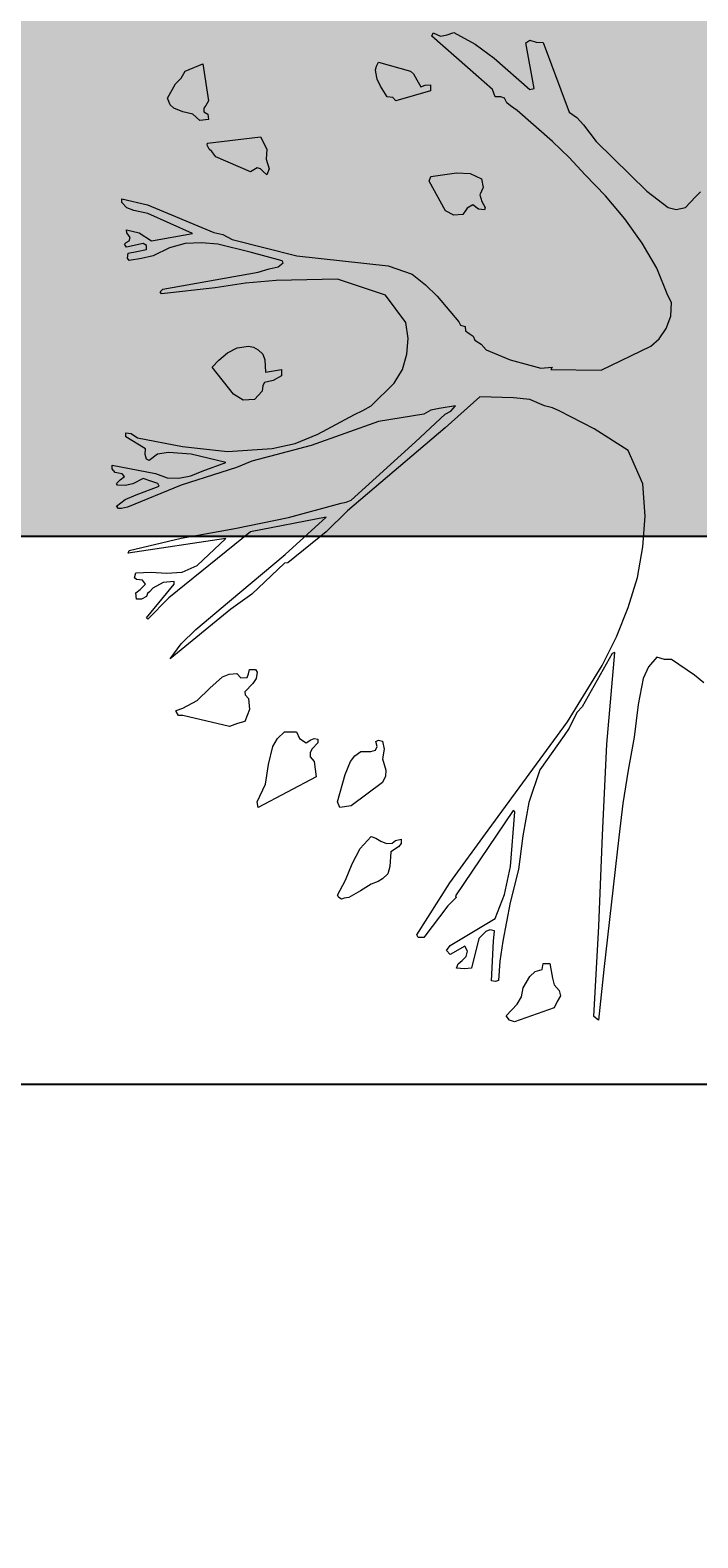
# Model space of a CAD drawing. Units: inches. Extents: x 84 to 1044, y -280 to 906.
# Tile 27 of 105: x 764 to 775, y -129 to -105. Entities that reach past the tile are written whole.
import ezdxf

# ---------------------------------------------------------------- set-up
doc = ezdxf.new("R2010")
doc.units = ezdxf.units.IN
for name, color, linetype, lineweight in [('A-ANNO-DIMS', 2, 'Continuous', 18), ('C-PROP', 7, 'Continuous', 25), ('L-PLNT', 114, 'Continuous', 15)]:
    doc.layers.add(name, color=color, linetype=linetype, lineweight=lineweight)
doc.layers.add('L-PLNT-PATT', color=9, linetype='Continuous', lineweight=9, true_color=0xafd9aa)
doc.styles.get("Standard").update_dxf_attribs({"font": 'arial.ttf'})
doc.dimstyles.get("Standard").update_dxf_attribs({"dimtxt": 0.18, "dimasz": 0.18, "dimexe": 0.18, "dimexo": 0.0625, "dimgap": 0.09, "dimtad": 0, "dimtih": 1, "dimtoh": 1, "dimdec": 4, "dimzin": 0, "dimdsep": 46, "dimtxsty": 'Standard', "dimcen": 0.09, "dimadec": 0, "dimazin": 0, "dimtfac": 1, "dimtdec": 4, "dimtofl": 0, "dimtmove": 0, "dimatfit": 3, "dimfxl": 1, "dimtolj": 1, "dimtzin": 0, "dimarcsym": 0})

# ---------------------------------------------------------------- blocks, each defined once
blk = doc.blocks.new('A$C37E508DF')
for p, q in [((0.3456, 1.093), (0.3469, 1.0964)), ((0.3842, 1.0591), (0.3456, 1.093)), ((0.3469, 1.0964), (0.355, 1.093)), ((0.355, 1.093), (0.3619, 1.0943)), ((0.3619, 1.0943), (0.3692, 1.0968)), ((0.3692, 1.0968), (0.3923, 1.0844)), ((0.3923, 1.0844), (0.4129, 1.069)), ((0.4472, 1.0857), (0.4515, 1.0887)), ((0.4562, 1.0364), (0.4472, 1.0857)), ((0.4515, 1.0887), (0.4584, 1.0865)), ((0.4584, 1.0865), (0.4657, 1.0861)), ((0.4657, 1.0861), (0.4939, 1.0107)), ((0.0789, 1.0552), (0.0978, 1.063)), ((0.0978, 1.063), (0.1042, 1.0231)), ((0.2847, 1.0565), (0.2856, 1.0604)), ((0.2856, 1.0604), (0.2877, 1.0647)), ((0.2877, 1.0647), (0.3224, 1.0552)), ((0.4129, 1.069), (0.4515, 1.0351)), ((0.0682, 1.0415), (0.0746, 1.0475)), ((0.0746, 1.0475), (0.0789, 1.0552)), ((0.2851, 1.054), (0.2847, 1.0565)), ((0.2864, 1.0463), (0.2851, 1.054)), ((0.2899, 1.039), (0.2864, 1.0463)), ((0.3224, 1.0552), (0.3255, 1.0522)), ((0.3255, 1.0522), (0.3293, 1.0458)), ((0.3293, 1.0458), (0.3336, 1.0381)), ((0.4112, 1.0351), (0.3842, 1.0591)), ((0.0596, 1.0257), (0.0682, 1.0415)), ((0.2972, 1.0274), (0.2899, 1.039)), ((0.3032, 1.0265), (0.2972, 1.0274)), ((0.3439, 1.0338), (0.3066, 1.0231)), ((0.3336, 1.0381), (0.3383, 1.0398)), ((0.3383, 1.0398), (0.3439, 1.0402)), ((0.3439, 1.0402), (0.3439, 1.0338)), ((0.4138, 1.0274), (0.4112, 1.0351)), ((0.4202, 1.0274), (0.4138, 1.0274)), ((0.4241, 1.0257), (0.4202, 1.0274)), ((0.4515, 1.0351), (0.4562, 1.0364)), ((0.0626, 1.0188), (0.0596, 1.0257)), ((0.0665, 1.0149), (0.0626, 1.0188)), ((0.0763, 1.0111), (0.0665, 1.0149)), ((0.087, 1.0085), (0.0763, 1.0111)), ((0.1012, 1.018), (0.099, 1.0149)), ((0.099, 1.0149), (0.099, 1.0111)), ((0.099, 1.0111), (0.1033, 1.0085)), ((0.1042, 1.0231), (0.1012, 1.018)), ((0.3066, 1.0231), (0.3032, 1.0265)), ((0.4267, 1.0209), (0.4241, 1.0257)), ((0.4305, 1.0175), (0.4267, 1.0209)), ((0.4378, 1.0124), (0.4305, 1.0175)), ((0.476, 0.9789), (0.4378, 1.0124)), ((0.4939, 1.0107), (0.5021, 1.0051)), ((0.0948, 1.0016), (0.087, 1.0085)), ((0.1042, 1.0029), (0.0948, 1.0016)), ((0.1033, 1.0085), (0.1042, 1.0029)), ((0.5021, 1.0051), (0.5094, 0.9969)), ((0.5094, 0.9969), (0.5231, 0.9789)), ((0.1029, 0.9772), (0.1604, 0.9841)), ((0.1604, 0.9841), (0.1672, 0.9708)), ((0.4939, 0.9618), (0.476, 0.9789)), ((0.5231, 0.9789), (0.578, 0.9253)), ((0.1025, 0.9751), (0.1029, 0.9772)), ((0.1046, 0.9708), (0.1025, 0.9751)), ((0.1076, 0.9682), (0.1046, 0.9708)), ((0.1119, 0.9626), (0.1076, 0.9682)), ((0.1496, 0.9463), (0.1119, 0.9626)), ((0.1672, 0.9708), (0.1664, 0.9601)), ((0.5111, 0.9429), (0.4939, 0.9618)), ((0.1565, 0.9506), (0.1496, 0.9463)), ((0.1604, 0.9493), (0.1565, 0.9506)), ((0.1629, 0.9468), (0.1604, 0.9493)), ((0.1672, 0.9429), (0.1629, 0.9468)), ((0.1664, 0.9601), (0.1698, 0.9493)), ((0.1698, 0.9493), (0.1672, 0.9429)), ((0.3426, 0.936), (0.3443, 0.9412)), ((0.3602, 0.9039), (0.3426, 0.936)), ((0.3443, 0.9412), (0.3722, 0.9451)), ((0.3722, 0.9451), (0.3868, 0.9446)), ((0.3868, 0.9446), (0.3992, 0.9386)), ((0.4009, 0.9292), (0.3975, 0.9215)), ((0.3992, 0.9386), (0.4009, 0.9292)), ((0.5334, 0.9202), (0.5111, 0.9429)), ((0.0103, 0.9129), (0.0103, 0.9172)), ((0.0103, 0.9172), (0.0382, 0.9107)), ((0.0159, 0.9073), (0.0103, 0.9129)), ((0.3975, 0.9215), (0.3996, 0.9142)), ((0.3996, 0.9142), (0.4031, 0.9077)), ((0.554, 0.8953), (0.5334, 0.9202)), ((0.578, 0.9253), (0.6011, 0.9077)), ((0.6196, 0.9077), (0.6303, 0.9189)), ((0.6303, 0.9189), (0.6359, 0.9245)), ((0.0232, 0.9043), (0.0159, 0.9073)), ((0.0386, 0.9013), (0.0232, 0.9043)), ((0.0382, 0.9107), (0.1098, 0.8807)), ((0.0866, 0.8794), (0.0386, 0.9013)), ((0.3692, 0.8992), (0.3602, 0.9039)), ((0.379, 0.9), (0.3692, 0.8992)), ((0.3838, 0.9069), (0.379, 0.9)), ((0.3898, 0.9107), (0.3838, 0.9069)), ((0.3958, 0.906), (0.3898, 0.9107)), ((0.4026, 0.9052), (0.3958, 0.906)), ((0.4031, 0.9077), (0.4026, 0.9052)), ((0.6011, 0.9077), (0.6097, 0.9056)), ((0.6097, 0.9056), (0.6196, 0.9077)), ((0.0159, 0.8803), (0.0154, 0.8837)), ((0.0154, 0.8837), (0.0292, 0.8803)), ((0.0176, 0.8777), (0.0159, 0.8803)), ((0.0292, 0.8803), (0.0424, 0.8717)), ((0.1098, 0.8807), (0.1196, 0.8786)), ((0.5728, 0.8691), (0.554, 0.8953)), ((0.0133, 0.8679), (0.015, 0.87)), ((0.0154, 0.8649), (0.0133, 0.8679)), ((0.015, 0.87), (0.0184, 0.8717)), ((0.0334, 0.8687), (0.0154, 0.8649)), ((0.0193, 0.8752), (0.0176, 0.8777)), ((0.0184, 0.8717), (0.0193, 0.8752)), ((0.0369, 0.8666), (0.0334, 0.8687)), ((0.0369, 0.8623), (0.0369, 0.8666)), ((0.0424, 0.8717), (0.0866, 0.8794)), ((0.0617, 0.864), (0.0442, 0.8554)), ((0.0789, 0.8687), (0.0617, 0.864)), ((0.0965, 0.8696), (0.0789, 0.8687)), ((0.1141, 0.8679), (0.0965, 0.8696)), ((0.1492, 0.8593), (0.1141, 0.8679)), ((0.1196, 0.8786), (0.1295, 0.873)), ((0.1295, 0.873), (0.1994, 0.8554)), ((0.5887, 0.8421), (0.5728, 0.8691)), ((0.0163, 0.8529), (0.0171, 0.8584)), ((0.0184, 0.8503), (0.0163, 0.8529)), ((0.0171, 0.8584), (0.0266, 0.8602)), ((0.0317, 0.8524), (0.0184, 0.8503)), ((0.0266, 0.8602), (0.0369, 0.8623)), ((0.0442, 0.8554), (0.0317, 0.8524)), ((0.1835, 0.8499), (0.1492, 0.8593)), ((0.1792, 0.8434), (0.1848, 0.8477)), ((0.1848, 0.8477), (0.1835, 0.8499)), ((0.1994, 0.8554), (0.2984, 0.8447)), ((0.0545, 0.8194), (0.1578, 0.8378)), ((0.1578, 0.8378), (0.1698, 0.8413)), ((0.1698, 0.8413), (0.1792, 0.8434)), ((0.2984, 0.8447), (0.3242, 0.8357)), ((0.3242, 0.8357), (0.3387, 0.8241)), ((0.6007, 0.8125), (0.5887, 0.8421)), ((0.0519, 0.8164), (0.0545, 0.8194)), ((0.0532, 0.8143), (0.0519, 0.8164)), ((0.1111, 0.8207), (0.0532, 0.8143)), ((0.1441, 0.8258), (0.1111, 0.8207)), ((0.1771, 0.8288), (0.1441, 0.8258)), ((0.2436, 0.8301), (0.1771, 0.8288)), ((0.2954, 0.813), (0.2436, 0.8301)), ((0.3387, 0.8241), (0.3512, 0.8117)), ((0.3173, 0.7834), (0.2954, 0.813)), ((0.3512, 0.8117), (0.3748, 0.7842)), ((0.6046, 0.8048), (0.6007, 0.8125)), ((0.6037, 0.7903), (0.6046, 0.8048)), ((0.3199, 0.7662), (0.3173, 0.7834)), ((0.3748, 0.7842), (0.3765, 0.7804)), ((0.599, 0.777), (0.6037, 0.7903)), ((0.3186, 0.7491), (0.3199, 0.7662)), ((0.3765, 0.7804), (0.3816, 0.7791)), ((0.3816, 0.7791), (0.382, 0.7744)), ((0.382, 0.7744), (0.3859, 0.7714)), ((0.3859, 0.7714), (0.3902, 0.7684)), ((0.3902, 0.7684), (0.3919, 0.7641)), ((0.5913, 0.7658), (0.599, 0.777)), ((0.1153, 0.7427), (0.1244, 0.7504)), ((0.1244, 0.7504), (0.1351, 0.7559)), ((0.1351, 0.7559), (0.1471, 0.7577)), ((0.1471, 0.7577), (0.1527, 0.7568)), ((0.1527, 0.7568), (0.1578, 0.7538)), ((0.1578, 0.7538), (0.1629, 0.7491)), ((0.3919, 0.7641), (0.3988, 0.7598)), ((0.3988, 0.7598), (0.4043, 0.7538)), ((0.4043, 0.7538), (0.4301, 0.7431)), ((0.5287, 0.7319), (0.5823, 0.7577)), ((0.5823, 0.7577), (0.5913, 0.7658)), ((0.1081, 0.7349), (0.1153, 0.7427)), ((0.1312, 0.7058), (0.1081, 0.7349)), ((0.1629, 0.7491), (0.1651, 0.7431)), ((0.1651, 0.7431), (0.1655, 0.7298)), ((0.3139, 0.7324), (0.3186, 0.7491)), ((0.4301, 0.7431), (0.4515, 0.7371)), ((0.4515, 0.7371), (0.4635, 0.7341)), ((0.4635, 0.7341), (0.4755, 0.7349)), ((0.4755, 0.7349), (0.4742, 0.7324)), ((0.1646, 0.7186), (0.1629, 0.7152)), ((0.1741, 0.7208), (0.1646, 0.7186)), ((0.1655, 0.7298), (0.1831, 0.7324)), ((0.1831, 0.7255), (0.1741, 0.7208)), ((0.1831, 0.7324), (0.1831, 0.7255)), ((0.28, 0.6933), (0.3049, 0.7178)), ((0.3049, 0.7178), (0.3139, 0.7324)), ((0.4742, 0.7324), (0.5287, 0.7319)), ((0.1415, 0.6994), (0.1312, 0.7058)), ((0.1621, 0.7092), (0.1539, 0.7002)), ((0.1629, 0.7152), (0.1621, 0.7092)), ((0.3975, 0.7028), (0.3598, 0.6693)), ((0.4339, 0.7019), (0.3975, 0.7028)), ((0.4515, 0.7002), (0.4339, 0.7019)), ((0.1539, 0.7002), (0.1415, 0.6994)), ((0.262, 0.6839), (0.271, 0.6882)), ((0.271, 0.6882), (0.28, 0.6933)), ((0.3443, 0.6886), (0.337, 0.6843)), ((0.3533, 0.6903), (0.3443, 0.6886)), ((0.3709, 0.6933), (0.3533, 0.6903)), ((0.3598, 0.6843), (0.3662, 0.6873)), ((0.3662, 0.6873), (0.3709, 0.6933)), ((0.4674, 0.6933), (0.4515, 0.7002)), ((0.476, 0.6912), (0.4674, 0.6933)), ((0.4832, 0.6878), (0.476, 0.6912)), ((0.521, 0.6685), (0.4832, 0.6878)), ((0.2877, 0.6762), (0.2152, 0.6505)), ((0.2221, 0.6625), (0.262, 0.6839)), ((0.3598, 0.6693), (0.2543, 0.5797)), ((0.337, 0.6843), (0.2877, 0.6762)), ((0.328, 0.6543), (0.3598, 0.6843)), ((0.5578, 0.6449), (0.521, 0.6685)), ((0.0146, 0.6599), (0.0146, 0.6642)), ((0.0146, 0.6642), (0.0206, 0.6633)), ((0.036, 0.6466), (0.0146, 0.6599)), ((0.0206, 0.6633), (0.0274, 0.6586)), ((0.0274, 0.6586), (0.0759, 0.6492)), ((0.1728, 0.647), (0.1977, 0.6526)), ((0.1977, 0.6526), (0.2221, 0.6625)), ((0.2581, 0.5913), (0.328, 0.6543)), ((0.0356, 0.6406), (0.036, 0.6466)), ((0.0369, 0.6355), (0.0356, 0.6406)), ((0.0489, 0.641), (0.0399, 0.6342)), ((0.0609, 0.6428), (0.0489, 0.641)), ((0.0853, 0.641), (0.0609, 0.6428)), ((0.0759, 0.6492), (0.1244, 0.644)), ((0.1226, 0.632), (0.0853, 0.641)), ((0.1244, 0.644), (0.1728, 0.647)), ((0.2152, 0.6505), (0.1509, 0.6333)), ((0.5737, 0.6089), (0.5578, 0.6449)), ((0, 0.629), (0.0467, 0.62)), ((0, 0.6252), (0, 0.629)), ((0.003, 0.6213), (0, 0.6252)), ((0.0069, 0.6204), (0.003, 0.6213)), ((0.0107, 0.6196), (0.0069, 0.6204)), ((0.0133, 0.617), (0.0107, 0.6196)), ((0.0399, 0.6342), (0.0369, 0.6355)), ((0.0467, 0.62), (0.0592, 0.6153)), ((0.1175, 0.6213), (0.0746, 0.6076)), ((0.0849, 0.6175), (0.0973, 0.6226)), ((0.0973, 0.6226), (0.1226, 0.632)), ((0.1342, 0.6265), (0.1175, 0.6213)), ((0.1509, 0.6333), (0.1342, 0.6265)), ((0.0047, 0.6093), (0.0086, 0.6132)), ((0.0056, 0.6076), (0.0047, 0.6093)), ((0.0141, 0.6072), (0.0056, 0.6076)), ((0.0086, 0.6132), (0.0133, 0.617)), ((0.0223, 0.6089), (0.0141, 0.6072)), ((0.0746, 0.6076), (0.0163, 0.5836)), ((0.0334, 0.6145), (0.0223, 0.6089)), ((0.0257, 0.5969), (0.0506, 0.6063)), ((0.0416, 0.6119), (0.0334, 0.6145)), ((0.0493, 0.6093), (0.0416, 0.6119)), ((0.0506, 0.6063), (0.0493, 0.6093)), ((0.0592, 0.6153), (0.072, 0.6149)), ((0.072, 0.6149), (0.0849, 0.6175)), ((0.5763, 0.5741), (0.5737, 0.6089)), ((0.0047, 0.5849), (0.0141, 0.5921)), ((0.0141, 0.5921), (0.0257, 0.5969)), ((0.1904, 0.5724), (0.2474, 0.5879)), ((0.2474, 0.5879), (0.253, 0.5892)), ((0.253, 0.5892), (0.2581, 0.5913)), ((0.0069, 0.5823), (0.0047, 0.5849)), ((0.0099, 0.5823), (0.0069, 0.5823)), ((0.0163, 0.5836), (0.0099, 0.5823)), ((0.1325, 0.5608), (0.1904, 0.5724)), ((0.2311, 0.5729), (0.1496, 0.557)), ((0.1869, 0.5325), (0.2311, 0.5729)), ((0.2543, 0.5797), (0.2311, 0.557)), ((0.5737, 0.5407), (0.5763, 0.5741)), ((0.1496, 0.557), (0.0613, 0.4858)), ((0.0746, 0.5501), (0.1325, 0.5608)), ((0.2311, 0.557), (0.1899, 0.5235)), ((0.1226, 0.5497), (0.0171, 0.5338)), ((0.0184, 0.5368), (0.0746, 0.5501)), ((0.0917, 0.5205), (0.1226, 0.5497)), ((0.5677, 0.5077), (0.5737, 0.5407)), ((0.0171, 0.5338), (0.0184, 0.5368)), ((0.1269, 0.482), (0.1869, 0.5325)), ((0.1861, 0.5231), (0.1509, 0.4897)), ((0.1899, 0.5235), (0.1861, 0.5231)), ((0.024, 0.5072), (0.0253, 0.5128)), ((0.0262, 0.5055), (0.024, 0.5072)), ((0.0253, 0.5128), (0.042, 0.5133)), ((0.0326, 0.5047), (0.0262, 0.5055)), ((0.042, 0.5133), (0.0587, 0.5124)), ((0.0587, 0.5124), (0.0755, 0.5133)), ((0.0755, 0.5133), (0.0917, 0.5205)), ((0.5578, 0.4751), (0.5677, 0.5077)), ((0.0253, 0.491), (0.03, 0.4948)), ((0.0262, 0.4841), (0.0253, 0.491)), ((0.03, 0.4948), (0.036, 0.5004)), ((0.036, 0.5004), (0.0326, 0.5047)), ((0.0369, 0.4639), (0.0669, 0.5004)), ((0.0382, 0.4905), (0.0369, 0.4871)), ((0.0403, 0.4922), (0.0382, 0.4905)), ((0.0437, 0.4961), (0.0403, 0.4922)), ((0.0549, 0.5021), (0.0437, 0.4961)), ((0.0669, 0.5034), (0.0549, 0.5021)), ((0.0669, 0.5004), (0.0669, 0.5034)), ((0.1509, 0.4897), (0.1282, 0.4734)), ((0.0317, 0.4841), (0.0262, 0.4841)), ((0.0369, 0.4871), (0.0317, 0.4841)), ((0.0613, 0.4858), (0.0386, 0.4627)), ((0.1282, 0.4734), (0.0626, 0.4198)), ((0.0905, 0.4515), (0.1269, 0.482)), ((0.545, 0.4434), (0.5578, 0.4751)), ((0.0386, 0.4627), (0.0369, 0.4639)), ((0.0746, 0.4361), (0.0905, 0.4515)), ((0.5295, 0.4125), (0.545, 0.4434)), ((0.0626, 0.4198), (0.0746, 0.4361)), ((0.5403, 0.4254), (0.5081, 0.3679)), ((0.5347, 0.3276), (0.5433, 0.4266)), ((0.5433, 0.4266), (0.5403, 0.4254)), ((0.1471, 0.4035), (0.1484, 0.4082)), ((0.1484, 0.4082), (0.1548, 0.4082)), ((0.1548, 0.4082), (0.1565, 0.4052)), ((0.4922, 0.3516), (0.5295, 0.4125)), ((0.5797, 0.4112), (0.5741, 0.3983)), ((0.5887, 0.4215), (0.5797, 0.4112)), ((0.5969, 0.4189), (0.5887, 0.4215)), ((0.6046, 0.4189), (0.5969, 0.4189)), ((0.6295, 0.4022), (0.6046, 0.4189)), ((0.1055, 0.388), (0.1192, 0.4001)), ((0.1192, 0.4001), (0.1265, 0.4031)), ((0.1265, 0.4031), (0.1346, 0.4039)), ((0.1346, 0.4039), (0.1389, 0.3992)), ((0.1389, 0.3992), (0.1458, 0.3996)), ((0.1518, 0.3932), (0.1432, 0.3842)), ((0.1458, 0.3996), (0.1471, 0.4035)), ((0.1556, 0.3983), (0.1518, 0.3932)), ((0.1565, 0.4052), (0.1556, 0.3983)), ((0.5741, 0.3983), (0.5686, 0.3705)), ((0.6397, 0.3936), (0.6295, 0.4022)), ((0.0917, 0.3748), (0.1055, 0.388)), ((0.1432, 0.3842), (0.1436, 0.3808)), ((0.1436, 0.3808), (0.1471, 0.3769)), ((0.1471, 0.3769), (0.1484, 0.3649)), ((0.069, 0.364), (0.0763, 0.3662)), ((0.069, 0.3627), (0.069, 0.364)), ((0.0716, 0.3585), (0.069, 0.3627)), ((0.0763, 0.3662), (0.0917, 0.3748)), ((0.1484, 0.3649), (0.1432, 0.352)), ((0.5025, 0.3619), (0.4982, 0.3537)), ((0.5081, 0.3679), (0.5025, 0.3619)), ((0.5686, 0.3705), (0.5643, 0.3349)), ((0.0763, 0.3585), (0.0716, 0.3585)), ((0.1269, 0.3464), (0.0763, 0.3585)), ((0.1355, 0.3499), (0.1269, 0.3464)), ((0.1432, 0.352), (0.1355, 0.3499)), ((0.4065, 0.2345), (0.4922, 0.3516)), ((0.4939, 0.3447), (0.4884, 0.337)), ((0.4982, 0.3537), (0.4939, 0.3447)), ((0.1737, 0.325), (0.1788, 0.3336)), ((0.1788, 0.3336), (0.1861, 0.3409)), ((0.1861, 0.3409), (0.199, 0.3409)), ((0.199, 0.3409), (0.2024, 0.3336)), ((0.2024, 0.3336), (0.2097, 0.3289)), ((0.2097, 0.3289), (0.2148, 0.3323)), ((0.2148, 0.3323), (0.2182, 0.3336)), ((0.2221, 0.3289), (0.2161, 0.3224)), ((0.2182, 0.3336), (0.2221, 0.3327)), ((0.2221, 0.3327), (0.2221, 0.3289)), ((0.2851, 0.3302), (0.2877, 0.3319)), ((0.2864, 0.325), (0.2851, 0.3302)), ((0.2877, 0.3319), (0.292, 0.3306)), ((0.292, 0.3306), (0.2941, 0.322)), ((0.4884, 0.337), (0.4622, 0.2997)), ((0.53, 0.229), (0.5347, 0.3276)), ((0.5643, 0.3349), (0.5578, 0.2993)), ((0.1689, 0.3053), (0.1737, 0.325)), ((0.2161, 0.3224), (0.214, 0.3186)), ((0.214, 0.3186), (0.214, 0.3139)), ((0.214, 0.3139), (0.2182, 0.3087)), ((0.2577, 0.3087), (0.2624, 0.3147)), ((0.2624, 0.3147), (0.2689, 0.3194)), ((0.2689, 0.3194), (0.2796, 0.3194)), ((0.2796, 0.3194), (0.2847, 0.3211)), ((0.2847, 0.3211), (0.2864, 0.325)), ((0.2941, 0.322), (0.292, 0.3117)), ((0.292, 0.3117), (0.2959, 0.2993)), ((0.1655, 0.2843), (0.1689, 0.3053)), ((0.2182, 0.3087), (0.2204, 0.292)), ((0.2436, 0.265), (0.2517, 0.2946)), ((0.2517, 0.2946), (0.2577, 0.3087)), ((0.2959, 0.2993), (0.2954, 0.2928)), ((0.4622, 0.2997), (0.4502, 0.2645)), ((0.5578, 0.2993), (0.5518, 0.2633)), ((0.1565, 0.265), (0.1655, 0.2843)), ((0.2204, 0.292), (0.1578, 0.259)), ((0.292, 0.286), (0.2581, 0.2607)), ((0.2954, 0.2928), (0.292, 0.286)), ((0.1578, 0.259), (0.1565, 0.265)), ((0.2461, 0.259), (0.2436, 0.265)), ((0.4502, 0.2645), (0.4438, 0.2285)), ((0.5518, 0.2633), (0.5475, 0.2268)), ((0.2581, 0.2607), (0.2461, 0.259)), ((0.4335, 0.2556), (0.3709, 0.1634)), ((0.4305, 0.1951), (0.4352, 0.2543)), ((0.4352, 0.2543), (0.4335, 0.2556)), ((0.3649, 0.1775), (0.4065, 0.2345)), ((0.4438, 0.2285), (0.4391, 0.1921)), ((0.5261, 0.1308), (0.53, 0.229)), ((0.2594, 0.1981), (0.268, 0.2148)), ((0.268, 0.2148), (0.28, 0.2277)), ((0.28, 0.2277), (0.2851, 0.226)), ((0.2851, 0.226), (0.2903, 0.2225)), ((0.2903, 0.2225), (0.2963, 0.22)), ((0.2963, 0.22), (0.3027, 0.2204)), ((0.3096, 0.2165), (0.301, 0.211)), ((0.3027, 0.2204), (0.3061, 0.2234)), ((0.3061, 0.2234), (0.3122, 0.2247)), ((0.3122, 0.22), (0.3096, 0.2165)), ((0.3122, 0.2247), (0.3122, 0.22)), ((0.5475, 0.2268), (0.5313, 0.084)), ((0.2521, 0.1805), (0.2594, 0.1981)), ((0.301, 0.211), (0.3002, 0.1951)), ((0.2436, 0.1642), (0.2521, 0.1805)), ((0.292, 0.1818), (0.2873, 0.1788)), ((0.298, 0.1874), (0.292, 0.1818)), ((0.3002, 0.1951), (0.298, 0.1874)), ((0.4241, 0.1651), (0.4305, 0.1951)), ((0.4391, 0.1921), (0.4301, 0.1561)), ((0.2448, 0.1616), (0.2436, 0.1642)), ((0.2684, 0.1689), (0.2556, 0.1616)), ((0.28, 0.1762), (0.2684, 0.1689)), ((0.2873, 0.1788), (0.28, 0.1762)), ((0.3293, 0.1213), (0.3649, 0.1775)), ((0.3709, 0.1634), (0.3718, 0.1616)), ((0.4138, 0.1389), (0.4241, 0.1651)), ((0.2478, 0.1599), (0.2448, 0.1616)), ((0.2508, 0.1608), (0.2478, 0.1599)), ((0.2556, 0.1616), (0.2508, 0.1608)), ((0.3628, 0.1526), (0.337, 0.1183)), ((0.3692, 0.1591), (0.3628, 0.1526)), ((0.3718, 0.1616), (0.3692, 0.1591)), ((0.4301, 0.1561), (0.4224, 0.1145)), ((0.3653, 0.1098), (0.4138, 0.1389)), ((0.5205, 0.033), (0.5261, 0.1308)), ((0.3306, 0.1183), (0.3293, 0.1213)), ((0.337, 0.1183), (0.3306, 0.1183)), ((0.3962, 0.1175), (0.3885, 0.0853)), ((0.4039, 0.1248), (0.3962, 0.1175)), ((0.4082, 0.1269), (0.4039, 0.1248)), ((0.4134, 0.1256), (0.4082, 0.1269)), ((0.4099, 0.0716), (0.4121, 0.1145)), ((0.4121, 0.1145), (0.4134, 0.1256)), ((0.4224, 0.1145), (0.4189, 0.093)), ((0.3615, 0.1042), (0.3653, 0.1098)), ((0.3653, 0.0999), (0.3615, 0.1042)), ((0.3812, 0.1089), (0.3653, 0.0999)), ((0.3842, 0.1037), (0.3812, 0.1089)), ((0.3825, 0.0978), (0.3842, 0.1037)), ((0.3722, 0.0853), (0.3739, 0.09)), ((0.3808, 0.0845), (0.3722, 0.0853)), ((0.3739, 0.09), (0.3782, 0.0935)), ((0.3782, 0.0935), (0.3825, 0.0978)), ((0.3885, 0.0853), (0.3808, 0.0845)), ((0.4189, 0.093), (0.4176, 0.072)), ((0.4571, 0.0815), (0.4648, 0.084)), ((0.4648, 0.084), (0.4657, 0.0905)), ((0.4657, 0.0905), (0.473, 0.0905)), ((0.473, 0.0905), (0.476, 0.0746)), ((0.5313, 0.084), (0.5257, 0.0291)), ((0.4142, 0.0707), (0.4099, 0.0716)), ((0.4176, 0.072), (0.4142, 0.0707)), ((0.4442, 0.0639), (0.4515, 0.0763)), ((0.4515, 0.0763), (0.4571, 0.0815)), ((0.476, 0.0746), (0.4777, 0.0673)), ((0.4777, 0.0673), (0.4832, 0.0613)), ((0.4378, 0.0463), (0.4425, 0.0544)), ((0.4425, 0.0544), (0.4442, 0.0639)), ((0.4811, 0.0493), (0.4777, 0.0424)), ((0.4845, 0.0553), (0.4811, 0.0493)), ((0.4832, 0.0613), (0.4845, 0.0553)), ((0.4258, 0.0339), (0.4378, 0.0463)), ((0.4296, 0.0291), (0.4258, 0.0339)), ((0.4777, 0.0424), (0.4348, 0.0274)), ((0.5257, 0.0291), (0.5205, 0.033)), ((0.4348, 0.0274), (0.4296, 0.0291))]:
    blk.add_line(p, q)
blk = doc.blocks.new('*D60')
at = {"layer": 'A-ANNO-DIMS', "color": 0, "lineweight": -2, "transparency": 16777216}
for p, q in [((134.179, -121.942), (134.179, -180.64)), ((992.074, -121.942), (992.074, -180.64)), ((134.359, -180.46), (562.733, -180.46)), ((991.894, -180.46), (563.521, -180.46))]:
    blk.add_line(p, q, dxfattribs=at)
at = {"layer": 'A-ANNO-DIMS', "color": 0, "transparency": 16777216}
for points in [[(134.359, -180.43), (134.359, -180.49), (134.179, -180.46)], [(991.894, -180.43), (991.894, -180.49), (992.074, -180.46)]]:
    blk.add_solid(points, dxfattribs=at)
at = {"layer": 'Defpoints', "color": 0, "transparency": 16777216}
for p in [(134.179, -121.88), (992.074, -121.88), (992.074, -180.46)]:
    blk.add_point(p, dxfattribs=at)
at = {"layer": 'A-ANNO-DIMS', "color": 0, "transparency": 16777216, "insert": (563.127, -180.46), "char_height": 0.18, "attachment_point": 5}
blk.add_mtext('\\A1;857.9', dxfattribs=at)

msp = doc.modelspace()

# ---------------------------------------------------------------- hatches: boundary and pattern name
at = {"layer": 'L-PLNT-PATT', "transparency": 33554597}
h = msp.add_hatch(color=256, dxfattribs=at)
h.dxf.hatch_style = 1
h.paths.add_polyline_path([(791.074, 31.12), (791.074, 91.12), (743.074, 91.12), (674.074, 91.12), (674.074, 31.12), (650.074, 31.12), (650.074, -112.88), (983.074, -112.88), (983.074, -64.88), (791.074, -64.88)])

# ---------------------------------------------------------------- linework, layer by layer
at = {"layer": 'C-PROP'}
for points in [[(143.179, -121.88), (134.179, -121.88), (134.179, 856.12), (992.074, 856.12), (992.074, -121.88), (624.574, -121.88)], [(143.179, -112.88), (143.179, 847.12), (983.074, 847.12), (983.074, -112.88), (624.574, -112.88)]]:
    msp.add_lwpolyline(points, dxfattribs=at)

# ---------------------------------------------------------------- block references
at = {"layer": 'L-PLNT', "xscale": 15.19586232982809, "yscale": 15.19586232982809, "zscale": 15.19586232982809}
msp.add_blockref('A$C37E508DF', (765.534, -121.265), dxfattribs=at)

# ---------------------------------------------------------------- dimensions: what is measured, and where the dimension line sits
at = {"layer": 'A-ANNO-DIMS'}
dim = msp.add_linear_dim(base=(992.074, -180.46), p1=(134.179, -121.88), p2=(992.074, -121.88), dimstyle='Standard', override={"dimdec": 1, "dimlfac": 1, "dimrnd": 0, "dimzin": 0, "dimdsep": 46, "dimlunit": 2}, dxfattribs=at)
dim.commit()
dim.dimension.update_dxf_attribs({"geometry": '*D60', "text_midpoint": (563.127, -180.46)})

doc.saveas('drawing.dxf')
